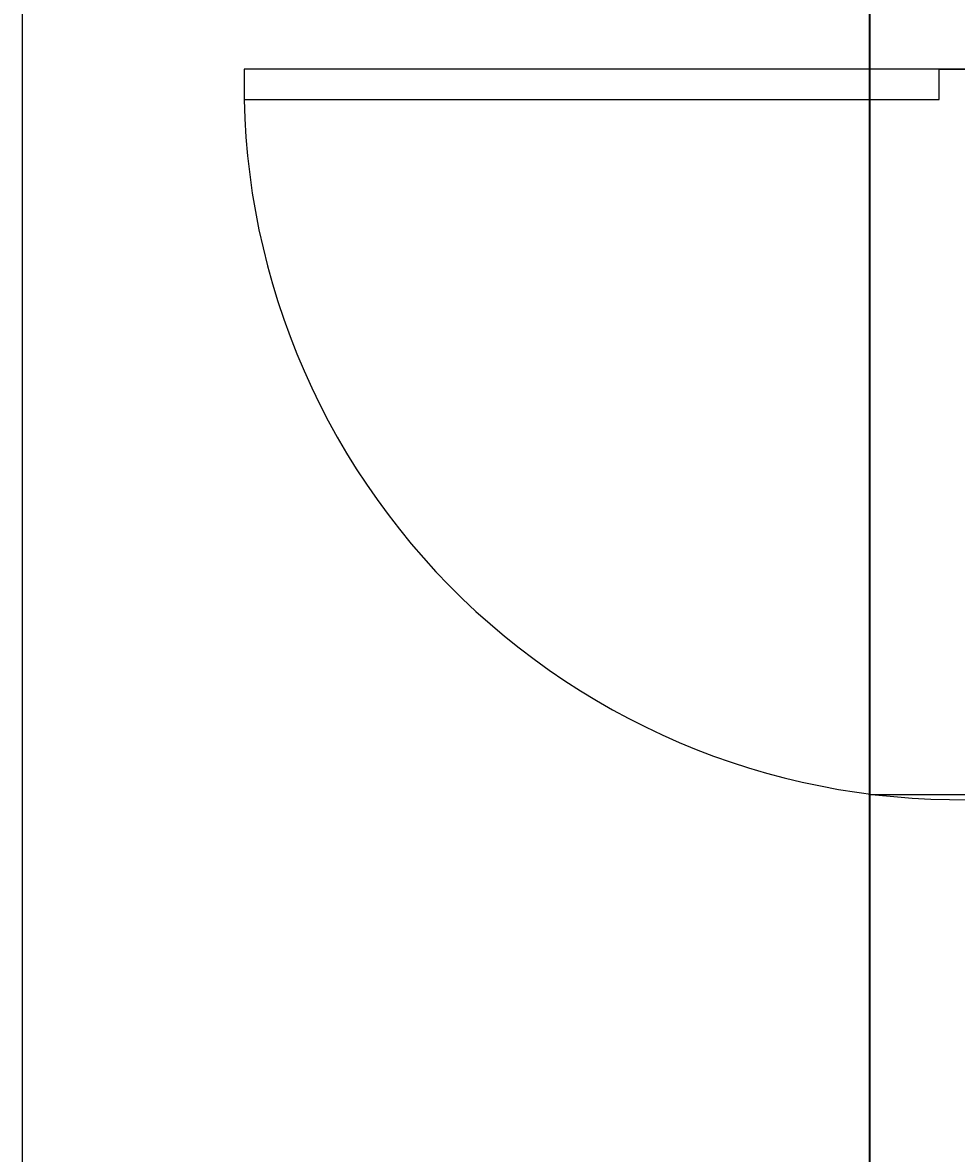
# Model space of a CAD drawing. Units: inches. Extents: x -61 to 1599, y -1316 to 257.
# Tile 140 of 204: x 492 to 540, y -74 to -16. Entities that reach past the tile are written whole.
import ezdxf

# ---------------------------------------------------------------- set-up
doc = ezdxf.new("R2010")
doc.units = ezdxf.units.IN
doc.header["$MEASUREMENT"] = 0
doc.linetypes.add('ACAD_ISO02W100', pattern=[15, 12, -3])
for name, color, linetype, lineweight in [('A-ANNO-DIMS', 2, 'Continuous', 18), ('A-WALL-JAMB', 4, 'ACAD_ISO02W100', 25), ('DOORS', 2, 'Continuous', 25), ('WALLS', 4, 'Continuous', 35)]:
    doc.layers.add(name, color=color, linetype=linetype, lineweight=lineweight)
doc.styles.get("Standard").update_dxf_attribs({"font": 'arial.ttf'})
doc.dimstyles.get("Standard").update_dxf_attribs({"dimtxt": 0.18, "dimasz": 0.18, "dimexe": 0.18, "dimexo": 0.0625, "dimgap": 0.09, "dimtad": 0, "dimtih": 1, "dimtoh": 1, "dimdec": 0, "dimzin": 0, "dimdsep": 46, "dimlunit": 3, "dimtxsty": 'Standard', "dimcen": 0.09, "dimadec": 0, "dimazin": 0, "dimtfac": 1, "dimtdec": 0, "dimtofl": 0, "dimtmove": 0, "dimatfit": 3, "dimfxl": 1, "dimtolj": 1, "dimtzin": 0, "dimarcsym": 0})

# ---------------------------------------------------------------- blocks, each defined once
blk = doc.blocks.new('DOOR-SWING-36')
blk.add_line((0, 0), (0, -5.4))
blk.add_lwpolyline([(0, 0), (0, 36), (-1.575, 36), (-1.575, 0)], close=True)
blk.add_arc((-0.739, -1.079), 37.088, 91.2913, 186.69053)
blk = doc.blocks.new('*D704')
at = {"layer": 'A-ANNO-DIMS', "color": 0, "lineweight": -2, "transparency": 16777216}
for p, q in [((491.833, -616.882), (491.833, 257.457)), ((492.013, 257.277), (517.874, 257.277)), ((544.523, 257.277), (518.661, 257.277)), ((544.703, -616.882), (544.703, 257.457))]:
    blk.add_line(p, q, dxfattribs=at)
at = {"layer": 'A-ANNO-DIMS', "color": 0, "transparency": 16777216}
for points in [[(492.013, 257.307), (492.013, 257.247), (491.833, 257.277)], [(544.523, 257.307), (544.523, 257.247), (544.703, 257.277)]]:
    blk.add_solid(points, dxfattribs=at)
at = {"layer": 'DEFPOINTS', "color": 0, "transparency": 16777216}
for p in [(544.703, 257.277), (491.833, -616.945), (544.703, -616.945)]:
    blk.add_point(p, dxfattribs=at)
at = {"layer": 'A-ANNO-DIMS', "color": 0, "transparency": 16777216, "insert": (518.268, 257.277), "char_height": 0.18, "attachment_point": 5}
blk.add_mtext('\\A1;52.87', dxfattribs=at)

msp = doc.modelspace()

# ---------------------------------------------------------------- linework, layer by layer
at = {"layer": 'A-WALL-JAMB'}
for p, q in [((544.7028, -18.1418), (535.7028, -18.1418)), ((544.7028, -55.7168), (535.7028, -55.7168))]:
    msp.add_line(p, q, dxfattribs=at)
at = {"layer": 'WALLS'}
msp.add_line((535.7028, -13.3229), (535.7028, -175.3229), dxfattribs=at)

# ---------------------------------------------------------------- block references
at = {"layer": 'DOORS', "rotation": 89.99999999999312}
msp.add_blockref('DOOR-SWING-36', (539.3028, -18.1418), dxfattribs=at)

# ---------------------------------------------------------------- dimensions: what is measured, and where the dimension line sits
at = {"layer": 'A-ANNO-DIMS'}
dim = msp.add_linear_dim(base=(544.7028, 257.2771), p1=(491.8327, -616.9446), p2=(544.7028, -616.9446), dimstyle='Standard', override={"dimdec": 2, "dimlfac": 1, "dimrnd": 0, "dimzin": 0, "dimdsep": 46, "dimlunit": 2}, dxfattribs=at)
dim.commit()
dim.dimension.update_dxf_attribs({"geometry": '*D704', "text_midpoint": (518.2677, 257.2771)})

doc.saveas('drawing.dxf')
